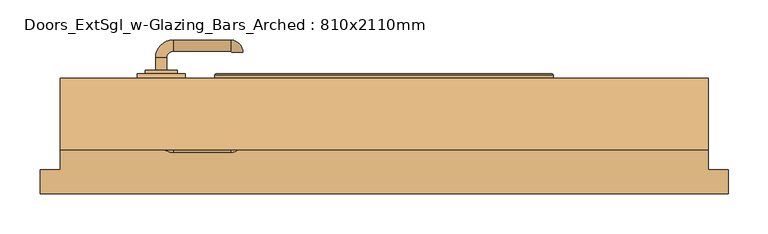
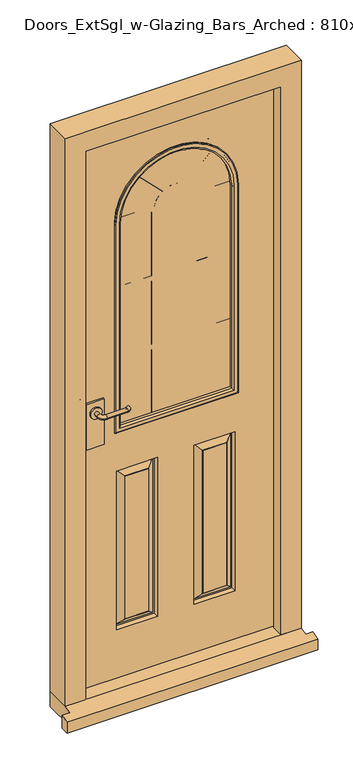
"""IFC4 building model written with IfcOpenShell, lengths in millimetres: door geometry, Doors_ExtSgl_w-Glazing_Bars_Arched : 810x2110mm."""

from ifc_helpers import new_model, si_unit, point, frame, frame_2d, origin, place, context, project, spatial, polyline, circle_curve, ellipse_curve, trimmed, segment, composite_curve, outline, extrude, faceted_brep, source, transform, mapped, element, save
from ifc_brep_helpers import plane_surface, cylinder_surface, revolved_surface, advanced_brep


def doors_extsgl_w_glazing_bars_arched_810x2110mm_84a0a083(model_context):
    return source(origin(), model_context, "Body", "SolidModel", [
        extrude(outline(composite_curve([segment(trimmed(circle_curve(frame_2d((1050.0, -278.5)), 20.0), [point((1050.0, -298.5))], [point((1050.0, -258.5))], False, "CARTESIAN"), True, "CONTINUOUS"), segment(trimmed(circle_curve(frame_2d((1050.0, -278.5)), 20.0), [point((1050.0, -258.5))], [point((1050.0, -298.5))], False, "CARTESIAN"), True, "CONTINUOUS")], self_intersect=False)), frame((0.0, 18.4, 0.0), z_axis=(0.0, 1.0, 0.0), x_axis=(0.0, 0.0, 1.0)), (0.0, 0.0, 1.0), 4.5929895),
        advanced_brep(
        [(-271.5, 22.9929895, 1050.0), (-285.5, 22.9929895, 1050.0), (-271.5, 38.4, 1050.0), (-285.5, 38.4, 1050.0), (-263.5, 60.4, 1050.0), (-263.5, 46.4, 1050.0), (-191.5, 46.4, 1050.0), (-191.5, 60.4, 1050.0), (-190.5, 45.4, 1050.0), (-176.5, 45.4, 1050.0)],
        [
            (0, 1, circle_curve(frame((-278.5, 22.9929895, 1050.0), z_axis=(0.0, -1.0, 0.0), x_axis=(-1.0, 0.0, 0.0)), 7.0)),
            (1, 0, circle_curve(frame((-278.5, 22.9929895, 1050.0), z_axis=(0.0, -1.0, 0.0), x_axis=(-1.0, 0.0, 0.0)), 7.0)),
            (0, 2),
            (2, 3, circle_curve(frame((-278.5, 38.4, 1050.0), z_axis=(0.0, -1.0, 0.0), x_axis=(-1.0, 0.0, 0.0)), 7.0)),
            (3, 1),
            (3, 2, circle_curve(frame((-278.5, 38.4, 1050.0), z_axis=(0.0, -1.0, 0.0), x_axis=(-1.0, 0.0, 0.0)), 7.0)),
            (4, 3, circle_curve(frame((-263.5, 38.4, 1050.0), z_axis=(0.0, 0.0, 1.0), x_axis=(-1.0, 0.0, 0.0)), 22.0)),
            (2, 5, circle_curve(frame((-263.5, 38.4, 1050.0), z_axis=(0.0, 0.0, -1.0), x_axis=(-1.0, 0.0, 0.0)), 8.0)),
            (5, 4, circle_curve(frame((-263.5, 53.4, 1050.0), z_axis=(-1.0, 0.0, 0.0), x_axis=(0.0, 1.0, 0.0)), 7.0)),
            (4, 5, circle_curve(frame((-263.5, 53.4, 1050.0), z_axis=(-1.0, 0.0, 0.0), x_axis=(0.0, 1.0, 0.0)), 7.0)),
            (5, 6),
            (6, 7, circle_curve(frame((-191.5, 53.4, 1050.0), z_axis=(-1.0, 0.0, 0.0), x_axis=(0.0, 1.0, 0.0)), 7.0)),
            (7, 4),
            (7, 6, circle_curve(frame((-191.5, 53.4, 1050.0), z_axis=(-1.0, 0.0, 0.0), x_axis=(0.0, 1.0, 0.0)), 7.0)),
            (8, 9, circle_curve(frame((-183.5, 45.4, 1050.0), z_axis=(0.0, -1.0, 0.0), x_axis=(1.0, 0.0, 0.0)), 7.0)),
            (9, 8, circle_curve(frame((-183.5, 45.4, 1050.0), z_axis=(0.0, -1.0, 0.0), x_axis=(1.0, 0.0, 0.0)), 7.0)),
            (9, 7, circle_curve(frame((-191.5, 45.4, 1050.0), z_axis=(0.0, 0.0, 1.0), x_axis=(0.0, 1.0, 0.0)), 15.0)),
            (6, 8, circle_curve(frame((-191.5, 45.4, 1050.0), z_axis=(0.0, 0.0, -1.0), x_axis=(0.0, 1.0, 0.0)), 1.0)),
        ],
        [
            plane_surface(frame((-278.5, 22.9929895, 1050.0), z_axis=(0.0, -1.0, 0.0), x_axis=(0.0, 0.0, 1.0))),
            cylinder_surface(frame((-278.5, 22.9929895, 1050.0), z_axis=(0.0, -1.0, 0.0), x_axis=(-1.0, 0.0, 0.0)), 7.0),
            revolved_surface(trimmed(ellipse_curve(frame((-278.5, 38.4, 1050.0), z_axis=(0.0, -1.0, 0.0), x_axis=(-1.0, 0.0, 0.0)), 7.0, 7.0), [point((-271.5, 38.4, 1050.0))], [point((-285.5, 38.4, 1050.0))], True, "CARTESIAN"), (-263.5, 38.4, 1050.0), (0.0, 0.0, -1.0)),
            revolved_surface(trimmed(ellipse_curve(frame((-278.5, 38.4, 1050.0), z_axis=(0.0, -1.0, 0.0), x_axis=(-1.0, 0.0, 0.0)), 7.0, 7.0), [point((-285.5, 38.4, 1050.0))], [point((-271.5, 38.4, 1050.0))], True, "CARTESIAN"), (-263.5, 38.4, 1050.0), (0.0, 0.0, -1.0)),
            cylinder_surface(frame((-263.5, 53.4, 1050.0), z_axis=(-1.0, 0.0, 0.0), x_axis=(0.0, 1.0, 0.0)), 7.0),
            plane_surface(frame((-183.5, 45.4, 1050.0), z_axis=(0.0, -1.0, 0.0), x_axis=(0.0, 0.0, 1.0))),
            revolved_surface(trimmed(ellipse_curve(frame((-191.5, 53.4, 1050.0), z_axis=(-1.0, 0.0, 0.0), x_axis=(0.0, 1.0, 0.0)), 7.0, 7.0), [point((-191.5, 46.4, 1050.0))], [point((-191.5, 60.4, 1050.0))], True, "CARTESIAN"), (-191.5, 45.4, 1050.0), (0.0, 0.0, -1.0)),
            revolved_surface(trimmed(ellipse_curve(frame((-191.5, 53.4, 1050.0), z_axis=(-1.0, 0.0, 0.0), x_axis=(0.0, 1.0, 0.0)), 7.0, 7.0), [point((-191.5, 60.4, 1050.0))], [point((-191.5, 46.4, 1050.0))], True, "CARTESIAN"), (-191.5, 45.4, 1050.0), (0.0, 0.0, -1.0)),
        ],
        [
            (0, [[1, 2]]),
            (1, [[-1, 3, 4, 5]]),
            (1, [[-2, -5, 6, -3]]),
            (2, [[7, -4, 8, 9]]),
            (3, [[-8, -6, -7, 10]]),
            (4, [[-9, 11, 12, 13]]),
            (4, [[-10, -13, 14, -11]]),
            (5, [[15, 16]]),
            (6, [[17, -12, 18, -16]]),
            (7, [[-18, -14, -17, -15]]),
        ],
    ),
        extrude(outline(polyline([(-248.5, 12.4), (-308.5, 12.4), (-308.5, 18.4), (-248.5, 18.4), (-248.5, 12.4)])), frame((0.0, 0.0, 925.0), z_axis=(0.0, 0.0, 1.0), x_axis=(1.0, 0.0, 0.0)), (0.0, 0.0, 1.0), 165.0),
        extrude(outline(composite_curve([segment(trimmed(circle_curve(frame_2d((1050.0, -278.5)), 20.0), [point((1050.0, -298.5))], [point((1050.0, -258.5))], False, "CARTESIAN"), True, "CONTINUOUS"), segment(trimmed(circle_curve(frame_2d((1050.0, -278.5)), 20.0), [point((1050.0, -258.5))], [point((1050.0, -298.5))], False, "CARTESIAN"), True, "CONTINUOUS")], self_intersect=False)), frame((0.0, -42.1929895, 0.0), z_axis=(0.0, 1.0, 0.0), x_axis=(0.0, 0.0, 1.0)), (0.0, 0.0, 1.0), 4.5929895),
        advanced_brep(
        [(-271.5, -42.1929895, 1050.0), (-285.5, -42.1929895, 1050.0), (-285.5, -57.6, 1050.0), (-271.5, -57.6, 1050.0), (-263.5, -79.6, 1050.0), (-263.5, -65.6, 1050.0), (-191.5, -79.6, 1050.0), (-191.5, -65.6, 1050.0), (-190.5, -64.6, 1050.0), (-176.5, -64.6, 1050.0)],
        [
            (0, 1, circle_curve(frame((-278.5, -42.1929895, 1050.0), z_axis=(0.0, 1.0, 0.0), x_axis=(-1.0, 0.0, 0.0)), 7.0)),
            (1, 0, circle_curve(frame((-278.5, -42.1929895, 1050.0), z_axis=(0.0, 1.0, 0.0), x_axis=(-1.0, 0.0, 0.0)), 7.0)),
            (1, 2),
            (2, 3, circle_curve(frame((-278.5, -57.6, 1050.0), z_axis=(0.0, 1.0, 0.0), x_axis=(-1.0, 0.0, 0.0)), 7.0)),
            (3, 0),
            (3, 2, circle_curve(frame((-278.5, -57.6, 1050.0), z_axis=(0.0, 1.0, 0.0), x_axis=(-1.0, 0.0, 0.0)), 7.0)),
            (4, 5, circle_curve(frame((-263.5, -72.6, 1050.0), z_axis=(-1.0, 0.0, 0.0), x_axis=(0.0, -1.0, 0.0)), 7.0)),
            (5, 3, circle_curve(frame((-263.5, -57.6, 1050.0), z_axis=(0.0, 0.0, -1.0), x_axis=(-1.0, 0.0, 0.0)), 8.0)),
            (2, 4, circle_curve(frame((-263.5, -57.6, 1050.0), z_axis=(0.0, 0.0, 1.0), x_axis=(-1.0, 0.0, 0.0)), 22.0)),
            (5, 4, circle_curve(frame((-263.5, -72.6, 1050.0), z_axis=(-1.0, 0.0, 0.0), x_axis=(0.0, -1.0, 0.0)), 7.0)),
            (4, 6),
            (6, 7, circle_curve(frame((-191.5, -72.6, 1050.0), z_axis=(-1.0, 0.0, 0.0), x_axis=(0.0, -1.0, 0.0)), 7.0)),
            (7, 5),
            (7, 6, circle_curve(frame((-191.5, -72.6, 1050.0), z_axis=(-1.0, 0.0, 0.0), x_axis=(0.0, -1.0, 0.0)), 7.0)),
            (8, 9, circle_curve(frame((-183.5, -64.6, 1050.0), z_axis=(0.0, 1.0, 0.0), x_axis=(1.0, 0.0, 0.0)), 7.0)),
            (9, 8, circle_curve(frame((-183.5, -64.6, 1050.0), z_axis=(0.0, 1.0, 0.0), x_axis=(1.0, 0.0, 0.0)), 7.0)),
            (8, 7, circle_curve(frame((-191.5, -64.6, 1050.0), z_axis=(0.0, 0.0, -1.0), x_axis=(0.0, -1.0, 0.0)), 1.0)),
            (6, 9, circle_curve(frame((-191.5, -64.6, 1050.0), z_axis=(0.0, 0.0, 1.0), x_axis=(0.0, -1.0, 0.0)), 15.0)),
        ],
        [
            plane_surface(frame((-278.5, -42.1929895, 1050.0), z_axis=(0.0, 1.0, 0.0), x_axis=(0.0, 0.0, 1.0))),
            cylinder_surface(frame((-278.5, -42.1929895, 1050.0), z_axis=(0.0, 1.0, 0.0), x_axis=(-1.0, 0.0, 0.0)), 7.0),
            revolved_surface(trimmed(ellipse_curve(frame((-278.5, -57.6, 1050.0), z_axis=(0.0, -1.0, 0.0), x_axis=(-1.0, 0.0, 0.0)), 7.0, 7.0), [point((-271.5, -57.6, 1050.0))], [point((-285.5, -57.6, 1050.0))], True, "CARTESIAN"), (-263.5, -57.6, 1050.0), (0.0, 0.0, -1.0)),
            revolved_surface(trimmed(ellipse_curve(frame((-278.5, -57.6, 1050.0), z_axis=(0.0, -1.0, 0.0), x_axis=(-1.0, 0.0, 0.0)), 7.0, 7.0), [point((-285.5, -57.6, 1050.0))], [point((-271.5, -57.6, 1050.0))], True, "CARTESIAN"), (-263.5, -57.6, 1050.0), (0.0, 0.0, -1.0)),
            cylinder_surface(frame((-263.5, -72.6, 1050.0), z_axis=(-1.0, 0.0, 0.0), x_axis=(0.0, -1.0, 0.0)), 7.0),
            plane_surface(frame((-183.5, -64.6, 1050.0), z_axis=(0.0, 1.0, 0.0), x_axis=(0.0, 0.0, 1.0))),
            revolved_surface(trimmed(ellipse_curve(frame((-191.5, -72.6, 1050.0), z_axis=(1.0, 0.0, 0.0), x_axis=(0.0, -1.0, 0.0)), 7.0, 7.0), [point((-191.5, -65.6, 1050.0))], [point((-191.5, -79.6, 1050.0))], True, "CARTESIAN"), (-191.5, -64.6, 1050.0), (0.0, 0.0, -1.0)),
            revolved_surface(trimmed(ellipse_curve(frame((-191.5, -72.6, 1050.0), z_axis=(1.0, 0.0, 0.0), x_axis=(0.0, -1.0, 0.0)), 7.0, 7.0), [point((-191.5, -79.6, 1050.0))], [point((-191.5, -65.6, 1050.0))], True, "CARTESIAN"), (-191.5, -64.6, 1050.0), (0.0, 0.0, -1.0)),
        ],
        [
            (0, [[1, 2]]),
            (1, [[3, 4, 5, -2]]),
            (1, [[-5, 6, -3, -1]]),
            (2, [[7, 8, -4, 9]]),
            (3, [[10, -9, -6, -8]]),
            (4, [[11, 12, 13, -7]]),
            (4, [[-13, 14, -11, -10]]),
            (5, [[15, 16]]),
            (6, [[-15, 17, -12, 18]]),
            (7, [[-16, -18, -14, -17]]),
        ],
    ),
        extrude(outline(polyline([(-248.5, -31.6), (-248.5, -37.6), (-308.5, -37.6), (-308.5, -31.6), (-248.5, -31.6)])), frame((0.0, 0.0, 925.0), z_axis=(0.0, 0.0, 1.0), x_axis=(1.0, 0.0, 0.0)), (0.0, 0.0, 1.0), 165.0),
        faceted_brep([(334.5, -76.6, 54.5), (334.5, -34.6, 54.5), (356.5, -34.6, 54.5), (356.5, 12.4, 54.5), (405.0, 12.4, 54.5), (405.0, -76.6, 54.5), (405.0, -76.6, 2110.0), (-405.0, -76.6, 2110.0), (-405.0, -76.6, 54.5), (-334.5, -76.6, 54.5), (-334.5, -76.6, 2039.5), (334.5, -76.6, 2039.5), (405.0, 12.4, 2110.0), (356.5, 12.4, 2061.5), (-356.5, 12.4, 2061.5), (-356.5, 12.4, 54.5), (-405.0, 12.4, 54.5), (-405.0, 12.4, 2110.0), (356.5, -34.6, 2061.5), (334.5, -34.6, 2039.5), (-334.5, -34.6, 2039.5), (-334.5, -34.6, 54.5), (-356.5, -34.6, 54.5), (-356.5, -34.6, 2061.5)], [[[0, 1, 2, 3, 4, 5]], [[5, 6, 7, 8, 9, 10, 11, 0]], [[4, 12, 6, 5]], [[3, 13, 14, 15, 16, 17, 12, 4]], [[2, 18, 13, 3]], [[1, 19, 20, 21, 22, 23, 18, 2]], [[0, 11, 19, 1]], [[9, 21, 20, 10]], [[8, 16, 15, 22, 21, 9]], [[7, 17, 16, 8]], [[14, 23, 22, 15]], [[6, 12, 17, 7]], [[13, 18, 23, 14]], [[10, 20, 19, 11]]]),
        advanced_brep(
        [(353.5, 12.4, 58.5), (-354.4250294, 12.4, 58.5), (-354.4250294, 12.4, 2058.5), (353.5, 12.4, 2058.5), (-203.5, 12.4, 958.5), (203.5, 12.4, 958.5), (203.5, 12.4, 1705.0), (-203.5, 12.4, 1705.0), (-62.5, 12.4, 808.5), (-203.5, 12.4, 808.5), (-203.5, 12.4, 233.5), (-62.5, 12.4, 233.5), (203.5, 12.4, 808.5), (62.5, 12.4, 808.5), (62.5, 12.4, 233.5), (203.5, 12.4, 233.5), (-92.5, 12.4, 263.5), (-173.5, 12.4, 263.5), (-173.5, 12.4, 778.5), (-92.5, 12.4, 778.5), (173.5, 12.4, 263.5), (92.5, 12.4, 263.5), (92.5, 12.4, 778.5), (173.5, 12.4, 778.5), (353.5, -31.6, 58.5), (353.5, -31.6, 2058.5), (-354.4250294, -31.6, 2058.5), (-354.4250294, -31.6, 58.5), (-203.5, -31.6, 958.5), (-203.5, -31.6, 1705.0), (203.5, -31.6, 1705.0), (203.5, -31.6, 958.5), (62.5, -31.6, 808.5), (203.5, -31.6, 808.5), (203.5, -31.6, 233.5), (62.5, -31.6, 233.5), (-203.5, -31.6, 808.5), (-62.5, -31.6, 808.5), (-62.5, -31.6, 233.5), (-203.5, -31.6, 233.5), (92.5, -31.6, 263.5), (173.5, -31.6, 263.5), (173.5, -31.6, 778.5), (92.5, -31.6, 778.5), (-173.5, -31.6, 263.5), (-92.5, -31.6, 263.5), (-92.5, -31.6, 778.5), (-173.5, -31.6, 778.5), (65.5, -16.6, 805.5), (65.5, -16.6, 236.5), (90.5, -30.6, 780.5), (70.5, -16.6, 800.5), (70.5, -16.6, 241.5), (90.5, -30.6, 261.5), (92.5, -30.6, 778.5), (92.5, -30.6, 263.5), (200.5, -16.6, 236.5), (195.5, -16.6, 241.5), (175.5, -30.6, 261.5), (173.5, -30.6, 263.5), (200.5, -16.6, 805.5), (195.5, -16.6, 800.5), (175.5, -30.6, 780.5), (173.5, -30.6, 778.5), (-200.5, -16.6, 805.5), (-200.5, -16.6, 236.5), (-175.5, -30.6, 780.5), (-195.5, -16.6, 800.5), (-195.5, -16.6, 241.5), (-175.5, -30.6, 261.5), (-173.5, -30.6, 778.5), (-173.5, -30.6, 263.5), (-65.5, -16.6, 236.5), (-70.5, -16.6, 241.5), (-90.5, -30.6, 261.5), (-92.5, -30.6, 263.5), (-65.5, -16.6, 805.5), (-70.5, -16.6, 800.5), (-90.5, -30.6, 780.5), (-92.5, -30.6, 778.5), (-92.5, 11.4, 263.5), (-92.5, 11.4, 778.5), (-70.5, -2.6, 241.5), (-90.5, 11.4, 261.5), (-90.5, 11.4, 780.5), (-70.5, -2.6, 800.5), (-65.5, -2.6, 236.5), (-65.5, -2.6, 805.5), (-173.5, 11.4, 778.5), (-175.5, 11.4, 780.5), (-195.5, -2.6, 800.5), (-200.5, -2.6, 805.5), (-173.5, 11.4, 263.5), (-175.5, 11.4, 261.5), (-195.5, -2.6, 241.5), (-200.5, -2.6, 236.5), (200.5, -2.6, 805.5), (200.5, -2.6, 236.5), (175.5, 11.4, 780.5), (195.5, -2.6, 800.5), (195.5, -2.6, 241.5), (175.5, 11.4, 261.5), (173.5, 11.4, 778.5), (173.5, 11.4, 263.5), (65.5, -2.6, 236.5), (70.5, -2.6, 241.5), (90.5, 11.4, 261.5), (92.5, 11.4, 263.5), (65.5, -2.6, 805.5), (70.5, -2.6, 800.5), (90.5, 11.4, 780.5), (92.5, 11.4, 778.5)],
        [
            (0, 1),
            (1, 2),
            (2, 3),
            (3, 0),
            (4, 5),
            (5, 6),
            (6, 7, circle_curve(frame((0.0, 12.4, 1705.0), z_axis=(0.0, -1.0, 0.0), x_axis=(1.0, 0.0, 0.0)), 203.5)),
            (7, 4),
            (8, 9),
            (9, 10),
            (10, 11),
            (11, 8),
            (12, 13),
            (13, 14),
            (14, 15),
            (15, 12),
            (16, 17),
            (17, 18),
            (18, 19),
            (19, 16),
            (20, 21),
            (21, 22),
            (22, 23),
            (23, 20),
            (24, 25),
            (25, 26),
            (26, 27),
            (27, 24),
            (28, 29),
            (29, 30, circle_curve(frame((0.0, -31.6, 1705.0), z_axis=(0.0, 1.0, 0.0), x_axis=(1.0, 0.0, 0.0)), 203.5)),
            (30, 31),
            (31, 28),
            (32, 33),
            (33, 34),
            (34, 35),
            (35, 32),
            (36, 37),
            (37, 38),
            (38, 39),
            (39, 36),
            (40, 41),
            (41, 42),
            (42, 43),
            (43, 40),
            (44, 45),
            (45, 46),
            (46, 47),
            (47, 44),
            (3, 25),
            (24, 0),
            (2, 26),
            (1, 27),
            (7, 29),
            (28, 4),
            (6, 30),
            (5, 31),
            (48, 32),
            (35, 49),
            (49, 48),
            (50, 51),
            (51, 52),
            (52, 53),
            (53, 50),
            (43, 54),
            (54, 55),
            (55, 40),
            (34, 56),
            (56, 49),
            (52, 57),
            (57, 58),
            (58, 53),
            (55, 59),
            (59, 41),
            (33, 60),
            (60, 56),
            (57, 61),
            (61, 62),
            (62, 58),
            (59, 63),
            (63, 42),
            (48, 60),
            (51, 61),
            (50, 62),
            (54, 63),
            (64, 36),
            (39, 65),
            (65, 64),
            (66, 67),
            (67, 68),
            (68, 69),
            (69, 66),
            (47, 70),
            (70, 71),
            (71, 44),
            (38, 72),
            (72, 65),
            (68, 73),
            (73, 74),
            (74, 69),
            (71, 75),
            (75, 45),
            (37, 76),
            (76, 72),
            (73, 77),
            (77, 78),
            (78, 74),
            (75, 79),
            (79, 46),
            (64, 76),
            (67, 77),
            (66, 78),
            (70, 79),
            (80, 16),
            (19, 81),
            (81, 80),
            (82, 83),
            (83, 84),
            (84, 85),
            (85, 82),
            (11, 86),
            (86, 87),
            (87, 8),
            (18, 88),
            (88, 81),
            (84, 89),
            (89, 90),
            (90, 85),
            (87, 91),
            (91, 9),
            (17, 92),
            (92, 88),
            (89, 93),
            (93, 94),
            (94, 90),
            (91, 95),
            (95, 10),
            (80, 92),
            (83, 93),
            (82, 94),
            (86, 95),
            (96, 12),
            (15, 97),
            (97, 96),
            (98, 99),
            (99, 100),
            (100, 101),
            (101, 98),
            (23, 102),
            (102, 103),
            (103, 20),
            (14, 104),
            (104, 97),
            (100, 105),
            (105, 106),
            (106, 101),
            (103, 107),
            (107, 21),
            (13, 108),
            (108, 104),
            (105, 109),
            (109, 110),
            (110, 106),
            (107, 111),
            (111, 22),
            (96, 108),
            (99, 109),
            (98, 110),
            (102, 111),
        ],
        [
            plane_surface(frame((353.5, 12.4, 58.5), z_axis=(0.0, 1.0, 0.0), x_axis=(0.0, 0.0, 1.0))),
            plane_surface(frame((353.5, -31.6, 58.5), z_axis=(0.0, -1.0, 0.0), x_axis=(0.0, 0.0, -1.0))),
            plane_surface(frame((353.5, 12.4, 58.5), z_axis=(1.0, 0.0, 0.0), x_axis=(0.0, -1.0, 0.0))),
            plane_surface(frame((353.5, 12.4, 2058.5), z_axis=(0.0, 0.0, 1.0), x_axis=(0.0, -1.0, 0.0))),
            plane_surface(frame((-354.4250294, 12.4, 2058.5), z_axis=(-1.0, 0.0, 0.0), x_axis=(0.0, -1.0, 0.0))),
            plane_surface(frame((-354.4250294, 12.4, 58.5), z_axis=(0.0, 0.0, -1.0), x_axis=(0.0, -1.0, 0.0))),
            plane_surface(frame((-203.5, 12.4, 958.5), z_axis=(1.0, 0.0, 0.0), x_axis=(0.0, -1.0, 0.0))),
            revolved_surface(polyline([(203.5, -31.6, 1705.0), (203.5, 12.4, 1705.0)]), (0.0, 12.4, 1705.0), (0.0, -1.0, 0.0)),
            plane_surface(frame((203.5, 12.4, 1705.0), z_axis=(-1.0, 0.0, 0.0), x_axis=(0.0, -1.0, 0.0))),
            plane_surface(frame((203.5, 12.4, 958.5), z_axis=(0.0, 0.0, 1.0), x_axis=(0.0, -1.0, 0.0))),
            plane_surface(frame((62.5, -31.6, 808.5), z_axis=(0.9805806756909202, -0.19611613513818407, 0.0), x_axis=(0.0, 0.0, -1.0))),
            plane_surface(frame((70.5, -16.6, 800.5), z_axis=(-0.5734623443633278, -0.8192319205190408, 0.0), x_axis=(0.0, 0.0, -1.0))),
            plane_surface(frame((92.5, -30.6, 778.5), z_axis=(-1.0, 0.0, 0.0), x_axis=(0.0, 0.0, -1.0))),
            plane_surface(frame((62.5, -31.6, 233.5), z_axis=(0.0, -0.19611613513818718, 0.9805806756909196), x_axis=(1.0, 0.0, 0.0))),
            plane_surface(frame((70.5, -16.6, 241.5), z_axis=(0.0, -0.8192319205190389, -0.5734623443633305), x_axis=(1.0, 0.0, 0.0))),
            plane_surface(frame((92.5, -30.6, 263.5), z_axis=(0.0, 0.0, -1.0), x_axis=(1.0, 0.0, 0.0))),
            plane_surface(frame((203.5, -31.6, 233.5), z_axis=(-0.9805806756909189, -0.19611613513819035, 0.0), x_axis=(0.0, 0.0, 1.0))),
            plane_surface(frame((195.5, -16.6, 241.5), z_axis=(0.5734623443633332, -0.819231920519037, 0.0), x_axis=(0.0, 0.0, 1.0))),
            plane_surface(frame((173.5, -30.6, 263.5), z_axis=(1.0, 0.0, 0.0), x_axis=(0.0, 0.0, 1.0))),
            plane_surface(frame((203.5, -31.6, 808.5), z_axis=(0.0, -0.19611613513818718, -0.9805806756909196), x_axis=(-1.0, 0.0, 0.0))),
            plane_surface(frame((200.5, -16.6, 805.5), z_axis=(0.0, -1.0, 0.0), x_axis=(-1.0, 0.0, 0.0))),
            plane_surface(frame((195.5, -16.6, 800.5), z_axis=(0.0, -0.8192319205190389, 0.5734623443633305), x_axis=(-1.0, 0.0, 0.0))),
            plane_surface(frame((175.5, -30.6, 780.5), z_axis=(0.0, -1.0, 0.0), x_axis=(-1.0, 0.0, 0.0))),
            plane_surface(frame((173.5, -30.6, 778.5), z_axis=(0.0, 0.0, 1.0), x_axis=(-1.0, 0.0, 0.0))),
            plane_surface(frame((-203.5, -31.6, 808.5), z_axis=(0.9805806756909202, -0.19611613513818407, 0.0), x_axis=(0.0, 0.0, -1.0))),
            plane_surface(frame((-195.5, -16.6, 800.5), z_axis=(-0.5734623443633278, -0.8192319205190408, 0.0), x_axis=(0.0, 0.0, -1.0))),
            plane_surface(frame((-173.5, -30.6, 778.5), z_axis=(-1.0, 0.0, 0.0), x_axis=(0.0, 0.0, -1.0))),
            plane_surface(frame((-203.5, -31.6, 233.5), z_axis=(0.0, -0.19611613513818724, 0.9805806756909196), x_axis=(1.0, 0.0, 0.0))),
            plane_surface(frame((-195.5, -16.6, 241.5), z_axis=(0.0, -0.819231920519039, -0.5734623443633305), x_axis=(1.0, 0.0, 0.0))),
            plane_surface(frame((-173.5, -30.6, 263.5), z_axis=(0.0, 0.0, -1.0), x_axis=(1.0, 0.0, 0.0))),
            plane_surface(frame((-62.5, -31.6, 233.5), z_axis=(-0.9805806756909189, -0.1961161351381904, 0.0), x_axis=(0.0, 0.0, 1.0))),
            plane_surface(frame((-70.5, -16.6, 241.5), z_axis=(0.5734623443633332, -0.8192319205190371, 0.0), x_axis=(0.0, 0.0, 1.0))),
            plane_surface(frame((-92.5, -30.6, 263.5), z_axis=(1.0, 0.0, 0.0), x_axis=(0.0, 0.0, 1.0))),
            plane_surface(frame((-62.5, -31.6, 808.5), z_axis=(0.0, -0.19611613513818724, -0.9805806756909196), x_axis=(-1.0, 0.0, 0.0))),
            plane_surface(frame((-65.5, -16.6, 805.5), z_axis=(0.0, -1.0, 0.0), x_axis=(-1.0, 0.0, 0.0))),
            plane_surface(frame((-70.5, -16.6, 800.5), z_axis=(0.0, -0.819231920519039, 0.5734623443633305), x_axis=(-1.0, 0.0, 0.0))),
            plane_surface(frame((-90.5, -30.6, 780.5), z_axis=(0.0, -1.0, 0.0), x_axis=(-1.0, 0.0, 0.0))),
            plane_surface(frame((-92.5, -30.6, 778.5), z_axis=(0.0, 0.0, 1.0), x_axis=(-1.0, 0.0, 0.0))),
            plane_surface(frame((-92.5, 12.4, 263.5), z_axis=(1.0, 0.0, 0.0), x_axis=(0.0, 0.0, 1.0))),
            plane_surface(frame((-90.5, 11.4, 261.5), z_axis=(0.5734623443633226, 0.8192319205190445, 0.0), x_axis=(0.0, 0.0, 1.0))),
            plane_surface(frame((-65.5, -2.6, 236.5), z_axis=(-0.9805806756909214, 0.1961161351381777, 0.0), x_axis=(0.0, 0.0, 1.0))),
            plane_surface(frame((-92.5, 12.4, 778.5), z_axis=(0.0, 0.0, 1.0), x_axis=(-1.0, 0.0, 0.0))),
            plane_surface(frame((-90.5, 11.4, 780.5), z_axis=(0.0, 0.8192319205190427, 0.5734623443633253), x_axis=(-1.0, 0.0, 0.0))),
            plane_surface(frame((-65.5, -2.6, 805.5), z_axis=(0.0, 0.19611613513818085, -0.9805806756909208), x_axis=(-1.0, 0.0, 0.0))),
            plane_surface(frame((-173.5, 12.4, 778.5), z_axis=(-1.0, 0.0, 0.0), x_axis=(0.0, 0.0, -1.0))),
            plane_surface(frame((-175.5, 11.4, 780.5), z_axis=(-0.5734623443633281, 0.8192319205190407, 0.0), x_axis=(0.0, 0.0, -1.0))),
            plane_surface(frame((-200.5, -2.6, 805.5), z_axis=(0.9805806756909202, 0.196116135138184, 0.0), x_axis=(0.0, 0.0, -1.0))),
            plane_surface(frame((-173.5, 12.4, 263.5), z_axis=(0.0, 0.0, -1.0), x_axis=(1.0, 0.0, 0.0))),
            plane_surface(frame((-173.5, 11.4, 263.5), z_axis=(0.0, 1.0, 0.0), x_axis=(1.0, 0.0, 0.0))),
            plane_surface(frame((-175.5, 11.4, 261.5), z_axis=(0.0, 0.8192319205190426, -0.5734623443633253), x_axis=(1.0, 0.0, 0.0))),
            plane_surface(frame((-195.5, -2.6, 241.5), z_axis=(0.0, 1.0, 0.0), x_axis=(1.0, 0.0, 0.0))),
            plane_surface(frame((-200.5, -2.6, 236.5), z_axis=(0.0, 0.19611613513818088, 0.9805806756909209), x_axis=(1.0, 0.0, 0.0))),
            plane_surface(frame((203.5, 12.4, 808.5), z_axis=(-0.9805806756909202, 0.19611613513818407, 0.0), x_axis=(0.0, 0.0, -1.0))),
            plane_surface(frame((195.5, -2.6, 800.5), z_axis=(0.5734623443633278, 0.8192319205190408, 0.0), x_axis=(0.0, 0.0, -1.0))),
            plane_surface(frame((173.5, 11.4, 778.5), z_axis=(1.0, 0.0, 0.0), x_axis=(0.0, 0.0, -1.0))),
            plane_surface(frame((203.5, 12.4, 233.5), z_axis=(0.0, 0.19611613513818724, 0.9805806756909196), x_axis=(-1.0, 0.0, 0.0))),
            plane_surface(frame((195.5, -2.6, 241.5), z_axis=(0.0, 0.819231920519039, -0.5734623443633305), x_axis=(-1.0, 0.0, 0.0))),
            plane_surface(frame((173.5, 11.4, 263.5), z_axis=(0.0, 0.0, -1.0), x_axis=(-1.0, 0.0, 0.0))),
            plane_surface(frame((62.5, 12.4, 233.5), z_axis=(0.9805806756909189, 0.19611613513819046, 0.0), x_axis=(0.0, 0.0, 1.0))),
            plane_surface(frame((70.5, -2.6, 241.5), z_axis=(-0.5734623443633331, 0.8192319205190371, 0.0), x_axis=(0.0, 0.0, 1.0))),
            plane_surface(frame((92.5, 11.4, 263.5), z_axis=(-1.0, 0.0, 0.0), x_axis=(0.0, 0.0, 1.0))),
            plane_surface(frame((62.5, 12.4, 808.5), z_axis=(0.0, 0.19611613513818724, -0.9805806756909196), x_axis=(1.0, 0.0, 0.0))),
            plane_surface(frame((65.5, -2.6, 805.5), z_axis=(0.0, 1.0, 0.0), x_axis=(1.0, 0.0, 0.0))),
            plane_surface(frame((70.5, -2.6, 800.5), z_axis=(0.0, 0.819231920519039, 0.5734623443633305), x_axis=(1.0, 0.0, 0.0))),
            plane_surface(frame((90.5, 11.4, 780.5), z_axis=(0.0, 1.0, 0.0), x_axis=(1.0, 0.0, 0.0))),
            plane_surface(frame((92.5, 11.4, 778.5), z_axis=(0.0, 0.0, 1.0), x_axis=(1.0, 0.0, 0.0))),
        ],
        [
            (0, [[1, 2, 3, 4], [5, 6, 7, 8], [9, 10, 11, 12], [13, 14, 15, 16]]),
            (0, [[17, 18, 19, 20]]),
            (0, [[21, 22, 23, 24]]),
            (1, [[25, 26, 27, 28], [29, 30, 31, 32], [33, 34, 35, 36], [37, 38, 39, 40]]),
            (1, [[41, 42, 43, 44]]),
            (1, [[45, 46, 47, 48]]),
            (2, [[49, -25, 50, -4]]),
            (3, [[51, -26, -49, -3]]),
            (4, [[52, -27, -51, -2]]),
            (5, [[-50, -28, -52, -1]]),
            (6, [[53, -29, 54, -8]]),
            (7, [[55, -30, -53, -7]]),
            (8, [[56, -31, -55, -6]]),
            (9, [[-54, -32, -56, -5]]),
            (10, [[57, -36, 58, 59]]),
            (11, [[60, 61, 62, 63]]),
            (12, [[-44, 64, 65, 66]]),
            (13, [[-35, 67, 68, -58]]),
            (14, [[69, 70, 71, -62]]),
            (15, [[72, 73, -41, -66]]),
            (16, [[-34, 74, 75, -67]]),
            (17, [[76, 77, 78, -70]]),
            (18, [[79, 80, -42, -73]]),
            (19, [[81, -74, -33, -57]]),
            (20, [[-68, -75, -81, -59], [82, -76, -69, -61]]),
            (21, [[83, -77, -82, -60]]),
            (22, [[-71, -78, -83, -63], [84, -79, -72, -65]]),
            (23, [[-43, -80, -84, -64]]),
            (24, [[85, -40, 86, 87]]),
            (25, [[88, 89, 90, 91]]),
            (26, [[-48, 92, 93, 94]]),
            (27, [[-39, 95, 96, -86]]),
            (28, [[97, 98, 99, -90]]),
            (29, [[100, 101, -45, -94]]),
            (30, [[-38, 102, 103, -95]]),
            (31, [[104, 105, 106, -98]]),
            (32, [[107, 108, -46, -101]]),
            (33, [[109, -102, -37, -85]]),
            (34, [[-96, -103, -109, -87], [110, -104, -97, -89]]),
            (35, [[111, -105, -110, -88]]),
            (36, [[-99, -106, -111, -91], [112, -107, -100, -93]]),
            (37, [[-47, -108, -112, -92]]),
            (38, [[113, -20, 114, 115]]),
            (39, [[116, 117, 118, 119]]),
            (40, [[-12, 120, 121, 122]]),
            (41, [[-19, 123, 124, -114]]),
            (42, [[125, 126, 127, -118]]),
            (43, [[128, 129, -9, -122]]),
            (44, [[-18, 130, 131, -123]]),
            (45, [[132, 133, 134, -126]]),
            (46, [[135, 136, -10, -129]]),
            (47, [[137, -130, -17, -113]]),
            (48, [[138, -132, -125, -117], [-124, -131, -137, -115]]),
            (49, [[139, -133, -138, -116]]),
            (50, [[140, -135, -128, -121], [-127, -134, -139, -119]]),
            (51, [[-11, -136, -140, -120]]),
            (52, [[141, -16, 142, 143]]),
            (53, [[144, 145, 146, 147]]),
            (54, [[-24, 148, 149, 150]]),
            (55, [[-15, 151, 152, -142]]),
            (56, [[153, 154, 155, -146]]),
            (57, [[156, 157, -21, -150]]),
            (58, [[-14, 158, 159, -151]]),
            (59, [[160, 161, 162, -154]]),
            (60, [[163, 164, -22, -157]]),
            (61, [[165, -158, -13, -141]]),
            (62, [[-152, -159, -165, -143], [166, -160, -153, -145]]),
            (63, [[167, -161, -166, -144]]),
            (64, [[-155, -162, -167, -147], [168, -163, -156, -149]]),
            (65, [[-23, -164, -168, -148]]),
        ],
    ),
        faceted_brep([(430.0, -131.6, 0.0), (430.0, -101.6, 0.0), (430.0, -101.6, 47.2703282), (430.0, -131.6, 38.5947221), (-430.0, -131.6, 38.5947221), (-430.0, -101.6, 47.2703282), (-430.0, -101.6, 0.0), (-430.0, -131.6, 0.0), (-405.0, -101.6, 0.0), (-405.0, 12.4, 0.0), (405.0, 12.4, 0.0), (405.0, -101.6, 0.0), (405.0, -101.6, 47.2703282), (405.0, -76.6, 54.5), (-405.0, -76.6, 54.5), (-405.0, -101.6, 47.2703282), (405.0, 12.4, 54.5), (-405.0, 12.4, 54.5)], [[[0, 1, 2, 3]], [[4, 5, 6, 7]], [[7, 6, 8, 9, 10, 11, 1, 0]], [[3, 4, 7, 0]], [[3, 2, 12, 13, 14, 15, 5, 4]], [[14, 13, 16, 17]], [[17, 16, 10, 9]], [[15, 14, 17, 9, 8]], [[8, 6, 5, 15]], [[11, 10, 16, 13, 12]], [[12, 2, 1, 11]]]),
        extrude(outline(composite_curve([segment(polyline([(958.5, -203.5), (958.5, 203.5), (1705.0, 203.5)]), True, "CONTINUOUS"), segment(trimmed(circle_curve(frame_2d((1705.0, 0.0)), 203.5), [point((1705.0, 203.5))], [point((1705.0, -203.5))], False, "CARTESIAN"), True, "CONTINUOUS"), segment(polyline([(1705.0, -203.5), (958.5, -203.5)]), True, "CONTINUOUS")], self_intersect=False)), frame((0.0, -21.6, 0.0), z_axis=(0.0, 1.0, 0.0), x_axis=(0.0, 0.0, 1.0)), (0.0, 0.0, 1.0), 24.0),
        advanced_brep(
        [(-211.5, -35.6, 950.5), (-211.5, -35.6, 1705.0), (-211.5, -31.6, 1705.0), (-211.5, -31.6, 950.5), (-209.5, -37.6, 952.5), (-209.5, -37.6, 1705.0), (-191.5, -32.6, 970.5), (-191.5, -32.6, 1705.0), (-196.5, -37.6, 1705.0), (-196.5, -37.6, 965.5), (-191.5, -21.6, 970.5), (-191.5, -21.6, 1705.0), (-203.5, -31.6, 958.5), (-203.5, -31.6, 1705.0), (-203.5, -21.6, 1705.0), (-203.5, -21.6, 958.5), (211.5, -35.6, 1705.0), (211.5, -31.6, 1705.0), (209.5, -37.6, 1705.0), (209.5, -37.6, 952.5), (196.5, -37.6, 1705.0), (196.5, -37.6, 965.5), (191.5, -32.6, 1705.0), (191.5, -21.6, 1705.0), (203.5, -21.6, 1705.0), (203.5, -21.6, 958.5), (191.5, -21.6, 970.5), (203.5, -31.6, 1705.0), (211.5, -31.6, 950.5), (203.5, -31.6, 958.5), (211.5, -35.6, 950.5), (191.5, -32.6, 970.5)],
        [
            (0, 1),
            (1, 2),
            (2, 3),
            (3, 0),
            (4, 5),
            (5, 1, circle_curve(frame((-209.5, -35.6, 1705.0), z_axis=(0.0, 0.0, -1.0), x_axis=(-1.0, 0.0, 0.0)), 2.0)),
            (0, 4, ellipse_curve(frame((-209.5, -35.6, 952.5), z_axis=(-0.7071067811865475, 0.0, 0.7071067811865475), x_axis=(-0.7071067811865472, 0.0, -0.7071067811865477)), 2.8284271, 2.0)),
            (6, 7),
            (7, 8, circle_curve(frame((-196.5, -32.6, 1705.0), z_axis=(0.0, 0.0, -1.0), x_axis=(-1.0, 0.0, 0.0)), 5.0)),
            (8, 9),
            (9, 6, ellipse_curve(frame((-196.5, -32.6, 965.5), z_axis=(-0.7071067811865475, 0.0, 0.7071067811865475), x_axis=(-0.7071067811865472, 0.0, -0.7071067811865477)), 7.0710678, 5.0)),
            (10, 11),
            (11, 7),
            (6, 10),
            (12, 13),
            (13, 14),
            (14, 15),
            (15, 12),
            (16, 17),
            (17, 2, circle_curve(frame((0.0, -31.6, 1705.0), z_axis=(0.0, -1.0, 0.0), x_axis=(-1.0, 0.0, 0.0)), 211.5)),
            (1, 16, circle_curve(frame((0.0, -35.6, 1705.0), z_axis=(0.0, 1.0, 0.0), x_axis=(-1.0, 0.0, 0.0)), 211.5)),
            (18, 16, circle_curve(frame((209.5, -35.6, 1705.0), z_axis=(0.0, 0.0, 1.0), x_axis=(1.0, 0.0, 0.0)), 2.0)),
            (5, 18, circle_curve(frame((0.0, -37.6, 1705.0), z_axis=(0.0, 1.0, 0.0), x_axis=(-1.0, 0.0, 0.0)), 209.5)),
            (4, 19),
            (19, 18),
            (20, 21),
            (21, 9),
            (8, 20, circle_curve(frame((0.0, -37.6, 1705.0), z_axis=(0.0, 1.0, 0.0), x_axis=(-1.0, 0.0, 0.0)), 196.5)),
            (22, 20, circle_curve(frame((196.5, -32.6, 1705.0), z_axis=(0.0, 0.0, 1.0), x_axis=(1.0, 0.0, 0.0)), 5.0)),
            (7, 22, circle_curve(frame((0.0, -32.6, 1705.0), z_axis=(0.0, 1.0, 0.0), x_axis=(-1.0, 0.0, 0.0)), 191.5)),
            (23, 22),
            (11, 23, circle_curve(frame((0.0, -21.6, 1705.0), z_axis=(0.0, 1.0, 0.0), x_axis=(-1.0, 0.0, 0.0)), 191.5)),
            (24, 25),
            (25, 15),
            (14, 24, circle_curve(frame((0.0, -21.6, 1705.0), z_axis=(0.0, 1.0, 0.0), x_axis=(-1.0, 0.0, 0.0)), 203.5)),
            (10, 26),
            (26, 23),
            (27, 24),
            (13, 27, circle_curve(frame((0.0, -31.6, 1705.0), z_axis=(0.0, 1.0, 0.0), x_axis=(-1.0, 0.0, 0.0)), 203.5)),
            (17, 28),
            (28, 3),
            (12, 29),
            (29, 27),
            (16, 30),
            (30, 28),
            (19, 30, ellipse_curve(frame((209.5, -35.6, 952.5), z_axis=(0.7071067811865475, 0.0, 0.7071067811865475), x_axis=(-0.7071067811865475, 0.0, 0.7071067811865476)), 2.8284271, 2.0)),
            (22, 31),
            (31, 21, ellipse_curve(frame((196.5, -32.6, 965.5), z_axis=(0.7071067811865475, 0.0, 0.7071067811865475), x_axis=(-0.7071067811865475, 0.0, 0.7071067811865476)), 7.0710678, 5.0)),
            (26, 31),
            (29, 25),
            (30, 0),
            (31, 6),
        ],
        [
            plane_surface(frame((-211.5, -31.6, 950.5), z_axis=(-1.0, 0.0, 0.0), x_axis=(0.0, 0.0, 1.0))),
            cylinder_surface(frame((-209.5, -35.6, 958.5), z_axis=(0.0, 0.0, -1.0), x_axis=(-1.0, 0.0, 0.0)), 2.0),
            cylinder_surface(frame((-196.5, -32.6, 958.5), z_axis=(0.0, 0.0, -1.0), x_axis=(-1.0, 0.0, 0.0)), 5.0),
            plane_surface(frame((-191.5, -32.6, 970.5), z_axis=(1.0, 0.0, 0.0), x_axis=(0.0, 0.0, 1.0))),
            plane_surface(frame((-203.5, -21.6, 958.5), z_axis=(-1.0, 0.0, 0.0), x_axis=(0.0, 0.0, 1.0))),
            cylinder_surface(frame((0.0, -31.6, 1705.0), z_axis=(0.0, -1.0, 0.0), x_axis=(-1.0, 0.0, 0.0)), 211.5),
            revolved_surface(trimmed(ellipse_curve(frame((-209.5, -35.6, 1705.0), z_axis=(0.0, 0.0, 1.0), x_axis=(-1.0, 0.0, 0.0)), 2.0, 2.0), [point((-211.5, -35.6, 1705.0))], [point((-209.5, -37.6, 1705.0))], True, "CARTESIAN"), (0.0, -31.6, 1705.0), (0.0, -1.0, 0.0)),
            plane_surface(frame((0.0, -37.6, 1705.0), z_axis=(0.0, -1.0, 0.0), x_axis=(-1.0, 0.0, 0.0))),
            revolved_surface(trimmed(ellipse_curve(frame((-196.5, -32.6, 1705.0), z_axis=(0.0, 0.0, 1.0), x_axis=(-1.0, 0.0, 0.0)), 5.0, 5.0), [point((-196.5, -37.6, 1705.0))], [point((-191.5, -32.6, 1705.0))], True, "CARTESIAN"), (0.0, -31.6, 1705.0), (0.0, -1.0, 0.0)),
            revolved_surface(polyline([(-191.5, -32.6, 1705.0), (-191.5, -21.6, 1705.0)]), (0.0, -31.6, 1705.0), (0.0, -1.0, 0.0)),
            plane_surface(frame((0.0, -21.6, 1705.0), z_axis=(0.0, 1.0, 0.0), x_axis=(-1.0, 0.0, 0.0))),
            cylinder_surface(frame((0.0, -31.6, 1705.0), z_axis=(0.0, -1.0, 0.0), x_axis=(-1.0, 0.0, 0.0)), 203.5),
            plane_surface(frame((0.0, -31.6, 1705.0), z_axis=(0.0, 1.0, 0.0), x_axis=(-1.0, 0.0, 0.0))),
            plane_surface(frame((211.5, -31.6, 1705.0), z_axis=(1.0, 0.0, 0.0), x_axis=(0.0, 0.0, -1.0))),
            cylinder_surface(frame((209.5, -35.6, 1705.0), z_axis=(0.0, 0.0, 1.0), x_axis=(1.0, 0.0, 0.0)), 2.0),
            cylinder_surface(frame((196.5, -32.6, 1705.0), z_axis=(0.0, 0.0, 1.0), x_axis=(1.0, 0.0, 0.0)), 5.0),
            plane_surface(frame((191.5, -32.6, 1705.0), z_axis=(-1.0, 0.0, 0.0), x_axis=(0.0, 0.0, -1.0))),
            plane_surface(frame((203.5, -21.6, 1705.0), z_axis=(1.0, 0.0, 0.0), x_axis=(0.0, 0.0, -1.0))),
            plane_surface(frame((211.5, -31.6, 950.5), z_axis=(0.0, 0.0, -1.0), x_axis=(-1.0, 0.0, 0.0))),
            cylinder_surface(frame((203.5, -35.6, 952.5), z_axis=(1.0, 0.0, 0.0), x_axis=(0.0, 0.0, -1.0)), 2.0),
            cylinder_surface(frame((203.5, -32.6, 965.5), z_axis=(1.0, 0.0, 0.0), x_axis=(0.0, 0.0, -1.0)), 5.0),
            plane_surface(frame((191.5, -32.6, 970.5), z_axis=(0.0, 0.0, 1.0), x_axis=(-1.0, 0.0, 0.0))),
            plane_surface(frame((203.5, -21.6, 958.5), z_axis=(0.0, 0.0, -1.0), x_axis=(-1.0, 0.0, 0.0))),
        ],
        [
            (0, [[1, 2, 3, 4]]),
            (1, [[5, 6, -1, 7]]),
            (2, [[8, 9, 10, 11]]),
            (3, [[12, 13, -8, 14]]),
            (4, [[15, 16, 17, 18]]),
            (5, [[19, 20, -2, 21]]),
            (6, [[22, -21, -6, 23]]),
            (7, [[-23, -5, 24, 25], [26, 27, -10, 28]]),
            (8, [[29, -28, -9, 30]]),
            (9, [[31, -30, -13, 32]]),
            (10, [[33, 34, -17, 35], [-32, -12, 36, 37]]),
            (11, [[38, -35, -16, 39]]),
            (12, [[40, 41, -3, -20], [-39, -15, 42, 43]]),
            (13, [[44, 45, -40, -19]]),
            (14, [[-25, 46, -44, -22]]),
            (15, [[47, 48, -26, -29]]),
            (16, [[-37, 49, -47, -31]]),
            (17, [[-43, 50, -33, -38]]),
            (18, [[51, -4, -41, -45]]),
            (19, [[-24, -7, -51, -46]]),
            (20, [[52, -11, -27, -48]]),
            (21, [[-36, -14, -52, -49]]),
            (22, [[-42, -18, -34, -50]]),
        ],
    ),
        advanced_brep(
        [(211.5, 16.4, 950.5), (211.5, 16.4, 1705.0), (211.5, 12.4, 1705.0), (211.5, 12.4, 950.5), (209.5, 18.4, 952.5), (209.5, 18.4, 1705.0), (191.5, 13.4, 970.5), (191.5, 13.4, 1705.0), (196.5, 18.4, 1705.0), (196.5, 18.4, 965.5), (191.5, 2.4, 970.5), (191.5, 2.4, 1705.0), (203.5, 12.4, 958.5), (203.5, 12.4, 1705.0), (203.5, 2.4, 1705.0), (203.5, 2.4, 958.5), (-211.5, 16.4, 1705.0), (-211.5, 12.4, 1705.0), (-209.5, 18.4, 1705.0), (-209.5, 18.4, 952.5), (-196.5, 18.4, 1705.0), (-196.5, 18.4, 965.5), (-191.5, 13.4, 1705.0), (-191.5, 2.4, 1705.0), (-203.5, 2.4, 1705.0), (-203.5, 2.4, 958.5), (-191.5, 2.4, 970.5), (-203.5, 12.4, 1705.0), (-211.5, 12.4, 950.5), (-203.5, 12.4, 958.5), (-211.5, 16.4, 950.5), (-191.5, 13.4, 970.5)],
        [
            (0, 1),
            (1, 2),
            (2, 3),
            (3, 0),
            (4, 5),
            (5, 1, circle_curve(frame((209.5, 16.4, 1705.0), z_axis=(0.0, 0.0, -1.0), x_axis=(1.0, 0.0, 0.0)), 2.0)),
            (0, 4, ellipse_curve(frame((209.5, 16.4, 952.5), z_axis=(0.7071067811865429, 0.0, 0.707106781186552), x_axis=(0.7071067811865519, 0.0, -0.707106781186543)), 2.8284271, 2.0)),
            (6, 7),
            (7, 8, circle_curve(frame((196.5, 13.4, 1705.0), z_axis=(0.0, 0.0, -1.0), x_axis=(1.0, 0.0, 0.0)), 5.0)),
            (8, 9),
            (9, 6, ellipse_curve(frame((196.5, 13.4, 965.5), z_axis=(0.7071067811865429, 0.0, 0.707106781186552), x_axis=(0.7071067811865519, 0.0, -0.707106781186543)), 7.0710678, 5.0)),
            (10, 11),
            (11, 7),
            (6, 10),
            (12, 13),
            (13, 14),
            (14, 15),
            (15, 12),
            (16, 17),
            (17, 2, circle_curve(frame((0.0, 12.4, 1705.0), z_axis=(0.0, 1.0, 0.0), x_axis=(1.0, 0.0, 0.0)), 211.5)),
            (1, 16, circle_curve(frame((0.0, 16.4, 1705.0), z_axis=(0.0, -1.0, 0.0), x_axis=(1.0, 0.0, 0.0)), 211.5)),
            (18, 16, circle_curve(frame((-209.5, 16.4, 1705.0), z_axis=(0.0, 0.0, 1.0), x_axis=(-1.0, 0.0, 0.0)), 2.0)),
            (5, 18, circle_curve(frame((0.0, 18.4, 1705.0), z_axis=(0.0, -1.0, 0.0), x_axis=(1.0, 0.0, 0.0)), 209.5)),
            (4, 19),
            (19, 18),
            (20, 21),
            (21, 9),
            (8, 20, circle_curve(frame((0.0, 18.4, 1705.0), z_axis=(0.0, -1.0, 0.0), x_axis=(1.0, 0.0, 0.0)), 196.5)),
            (22, 20, circle_curve(frame((-196.5, 13.4, 1705.0), z_axis=(0.0, 0.0, 1.0), x_axis=(-1.0, 0.0, 0.0)), 5.0)),
            (7, 22, circle_curve(frame((0.0, 13.4, 1705.0), z_axis=(0.0, -1.0, 0.0), x_axis=(1.0, 0.0, 0.0)), 191.5)),
            (23, 22),
            (11, 23, circle_curve(frame((0.0, 2.4, 1705.0), z_axis=(0.0, -1.0, 0.0), x_axis=(1.0, 0.0, 0.0)), 191.5)),
            (24, 25),
            (25, 15),
            (14, 24, circle_curve(frame((0.0, 2.4, 1705.0), z_axis=(0.0, -1.0, 0.0), x_axis=(1.0, 0.0, 0.0)), 203.5)),
            (10, 26),
            (26, 23),
            (27, 24),
            (13, 27, circle_curve(frame((0.0, 12.4, 1705.0), z_axis=(0.0, -1.0, 0.0), x_axis=(1.0, 0.0, 0.0)), 203.5)),
            (17, 28),
            (28, 3),
            (12, 29),
            (29, 27),
            (16, 30),
            (30, 28),
            (19, 30, ellipse_curve(frame((-209.5, 16.4, 952.5), z_axis=(-0.707106781186552, 0.0, 0.7071067811865429), x_axis=(0.7071067811865428, 0.0, 0.7071067811865521)), 2.8284271, 2.0)),
            (22, 31),
            (31, 21, ellipse_curve(frame((-196.5, 13.4, 965.5), z_axis=(-0.707106781186552, 0.0, 0.7071067811865429), x_axis=(0.7071067811865428, 0.0, 0.7071067811865521)), 7.0710678, 5.0)),
            (26, 31),
            (29, 25),
            (30, 0),
            (31, 6),
        ],
        [
            plane_surface(frame((211.5, 12.4, 950.5), z_axis=(1.0, 0.0, 0.0), x_axis=(0.0, 0.0, 1.0))),
            cylinder_surface(frame((209.5, 16.4, 958.5), z_axis=(0.0, 0.0, -1.0), x_axis=(1.0, 0.0, 0.0)), 2.0),
            cylinder_surface(frame((196.5, 13.4, 958.5), z_axis=(0.0, 0.0, -1.0), x_axis=(1.0, 0.0, 0.0)), 5.0),
            plane_surface(frame((191.5, 13.4, 970.5), z_axis=(-1.0, 0.0, 0.0), x_axis=(0.0, 0.0, 1.0))),
            plane_surface(frame((203.5, 2.4, 958.5), z_axis=(1.0, 0.0, 0.0), x_axis=(0.0, 0.0, 1.0))),
            cylinder_surface(frame((0.0, 12.4, 1705.0), z_axis=(0.0, 1.0, 0.0), x_axis=(1.0, 0.0, 0.0)), 211.5),
            revolved_surface(trimmed(ellipse_curve(frame((209.5, 16.4, 1705.0), z_axis=(0.0, 0.0, 1.0), x_axis=(1.0, 0.0, 0.0)), 2.0, 2.0), [point((211.5, 16.4, 1705.0))], [point((209.5, 18.4, 1705.0))], True, "CARTESIAN"), (0.0, 12.4, 1705.0), (0.0, 1.0, 0.0)),
            plane_surface(frame((0.0, 18.4, 1705.0), z_axis=(0.0, 1.0, 0.0), x_axis=(1.0, 0.0, 0.0))),
            revolved_surface(trimmed(ellipse_curve(frame((196.5, 13.4, 1705.0), z_axis=(0.0, 0.0, 1.0), x_axis=(1.0, 0.0, 0.0)), 5.0, 5.0), [point((196.5, 18.4, 1705.0))], [point((191.5, 13.4, 1705.0))], True, "CARTESIAN"), (0.0, 12.4, 1705.0), (0.0, 1.0, 0.0)),
            revolved_surface(polyline([(191.5, 13.4, 1705.0), (191.5, 2.4000000000000004, 1705.0)]), (0.0, 12.4, 1705.0), (0.0, 1.0, 0.0)),
            plane_surface(frame((0.0, 2.4, 1705.0), z_axis=(0.0, -1.0, 0.0), x_axis=(1.0, 0.0, 0.0))),
            cylinder_surface(frame((0.0, 12.4, 1705.0), z_axis=(0.0, 1.0, 0.0), x_axis=(1.0, 0.0, 0.0)), 203.5),
            plane_surface(frame((0.0, 12.4, 1705.0), z_axis=(0.0, -1.0, 0.0), x_axis=(1.0, 0.0, 0.0))),
            plane_surface(frame((-211.5, 12.4, 1705.0), z_axis=(-1.0, 0.0, 0.0), x_axis=(0.0, 0.0, -1.0))),
            cylinder_surface(frame((-209.5, 16.4, 1705.0), z_axis=(0.0, 0.0, 1.0), x_axis=(-1.0, 0.0, 0.0)), 2.0),
            cylinder_surface(frame((-196.5, 13.4, 1705.0), z_axis=(0.0, 0.0, 1.0), x_axis=(-1.0, 0.0, 0.0)), 5.0),
            plane_surface(frame((-191.5, 13.4, 1705.0), z_axis=(1.0, 0.0, 0.0), x_axis=(0.0, 0.0, -1.0))),
            plane_surface(frame((-203.5, 2.4, 1705.0), z_axis=(-1.0, 0.0, 0.0), x_axis=(0.0, 0.0, -1.0))),
            plane_surface(frame((-211.5, 12.4, 950.5), z_axis=(0.0, 0.0, -1.0), x_axis=(1.0, 0.0, 0.0))),
            cylinder_surface(frame((-203.5, 16.4, 952.5), z_axis=(-1.0, 0.0, 0.0), x_axis=(0.0, 0.0, -1.0)), 2.0),
            cylinder_surface(frame((-203.5, 13.4, 965.5), z_axis=(-1.0, 0.0, 0.0), x_axis=(0.0, 0.0, -1.0)), 5.0),
            plane_surface(frame((-191.5, 13.4, 970.5), z_axis=(0.0, 0.0, 1.0), x_axis=(1.0, 0.0, 0.0))),
            plane_surface(frame((-203.5, 2.4, 958.5), z_axis=(0.0, 0.0, -1.0), x_axis=(1.0, 0.0, 0.0))),
        ],
        [
            (0, [[1, 2, 3, 4]]),
            (1, [[5, 6, -1, 7]]),
            (2, [[8, 9, 10, 11]]),
            (3, [[12, 13, -8, 14]]),
            (4, [[15, 16, 17, 18]]),
            (5, [[19, 20, -2, 21]]),
            (6, [[22, -21, -6, 23]]),
            (7, [[-23, -5, 24, 25], [26, 27, -10, 28]]),
            (8, [[29, -28, -9, 30]]),
            (9, [[31, -30, -13, 32]]),
            (10, [[33, 34, -17, 35], [-32, -12, 36, 37]]),
            (11, [[38, -35, -16, 39]]),
            (12, [[40, 41, -3, -20], [-39, -15, 42, 43]]),
            (13, [[44, 45, -40, -19]]),
            (14, [[-25, 46, -44, -22]]),
            (15, [[47, 48, -26, -29]]),
            (16, [[-37, 49, -47, -31]]),
            (17, [[-43, 50, -33, -38]]),
            (18, [[51, -4, -41, -45]]),
            (19, [[-24, -7, -51, -46]]),
            (20, [[52, -11, -27, -48]]),
            (21, [[-36, -14, -52, -49]]),
            (22, [[-42, -18, -34, -50]]),
        ],
    ),
        extrude(outline(composite_curve([segment(polyline([(958.5, 57.8333333), (958.5, 77.8333333), (1197.3333333, 77.8333333), (1197.3333333, 203.5), (1217.3333333, 203.5), (1217.3333333, 77.8333333), (1446.1666667, 77.8333333), (1446.1666667, 203.5), (1466.1666667, 203.5), (1466.1666667, 77.8333333), (1695.0, 77.8333333), (1695.0, 203.5), (1715.0, 203.5), (1715.0, 67.8333333)]), True, "CONTINUOUS"), segment(trimmed(circle_curve(frame_2d((1702.0, 0.0)), 69.0678008), [point((1715.0, 67.8333333))], [point((1744.9484515, 54.0905872))], False, "CARTESIAN"), True, "CONTINUOUS"), segment(polyline([(1744.9484515, 54.0905872), (1841.6513208, 150.7934565)]), True, "CONTINUOUS"), segment(trimmed(circle_curve(frame_2d((1705.0, 0.0)), 203.5), [point((1841.6513208, 150.7934565))], [point((1855.7934565, 136.6513208))], False, "CARTESIAN"), True, "CONTINUOUS"), segment(polyline([(1855.7934565, 136.6513208), (1758.6513897, 39.5092541)]), True, "CONTINUOUS"), segment(trimmed(circle_curve(frame_2d((1702.0, 0.0)), 69.0678008), [point((1758.6513897, 39.5092541))], [point((1770.3400403, 10.0))], False, "CARTESIAN"), True, "CONTINUOUS"), segment(polyline([(1770.3400403, 10.0), (1908.2541512, 10.0)]), True, "CONTINUOUS"), segment(trimmed(circle_curve(frame_2d((1705.0, 0.0)), 203.5), [point((1908.2541512, 10.0))], [point((1908.2541512, -10.0))], False, "CARTESIAN"), True, "CONTINUOUS"), segment(polyline([(1908.2541512, -10.0), (1770.3400403, -10.0)]), True, "CONTINUOUS"), segment(trimmed(circle_curve(frame_2d((1702.0, 0.0)), 69.0678008), [point((1770.3400403, -10.0))], [point((1758.6513897, -39.5092541))], False, "CARTESIAN"), True, "CONTINUOUS"), segment(polyline([(1758.6513897, -39.5092541), (1855.7934565, -136.6513208)]), True, "CONTINUOUS"), segment(trimmed(circle_curve(frame_2d((1705.0, 0.0)), 203.5), [point((1855.7934565, -136.6513208))], [point((1841.6513208, -150.7934565))], False, "CARTESIAN"), True, "CONTINUOUS"), segment(polyline([(1841.6513208, -150.7934565), (1744.9484515, -54.0905872)]), True, "CONTINUOUS"), segment(trimmed(circle_curve(frame_2d((1702.0, 0.0)), 69.0678008), [point((1744.9484515, -54.0905872))], [point((1715.0, -67.8333333))], False, "CARTESIAN"), True, "CONTINUOUS"), segment(polyline([(1715.0, -67.8333333), (1715.0, -203.5), (1695.0, -203.5), (1695.0, -77.8333333), (1466.1666667, -77.8333333), (1466.1666667, -203.5), (1446.1666667, -203.5), (1446.1666667, -77.8333333), (1217.3333333, -77.8333333), (1217.3333333, -203.5), (1197.3333333, -203.5), (1197.3333333, -77.8333333), (958.5, -77.8333333), (958.5, -57.8333333), (1197.3333333, -57.8333333), (1197.3333333, 57.8333333), (958.5, 57.8333333)]), True, "CONTINUOUS")], self_intersect=False), holes=[polyline([(1695.0, 57.8333333), (1466.1666667, 57.8333333), (1466.1666667, -57.8333333), (1695.0, -57.8333333), (1695.0, 57.8333333)]), polyline([(1446.1666667, -57.8333333), (1446.1666667, 57.8333333), (1217.3333333, 57.8333333), (1217.3333333, -57.8333333), (1446.1666667, -57.8333333)])]), frame((0.0, -21.6, 0.0), z_axis=(0.0, 1.0, 0.0), x_axis=(0.0, 0.0, 1.0)), (0.0, 0.0, 1.0), 24.0),
    ])


if __name__ == "__main__":
    model = new_model("IFC4")
    model_context = context("Model", 3, world=origin())
    ifc_project = project(units=[si_unit("LENGTHUNIT", "METRE", prefix="MILLI")], contexts=[model_context])
    site = spatial("IfcSite", under=ifc_project)
    building = spatial("IfcBuilding", under=site)
    placement = place(None, origin())
    doors_extsgl_w_glazing_bars_arched_810x2110mm_shape = doors_extsgl_w_glazing_bars_arched_810x2110mm_84a0a083(model_context)
    element("IfcDoor", 1, ObjectType="Doors_ExtSgl_w-Glazing_Bars_Arched : 810x2110mm", at=placement, inside=building, context=model_context, shape_type="MappedRepresentation", body=[
        mapped(doors_extsgl_w_glazing_bars_arched_810x2110mm_shape, transform((0.0, 0.0, 0.0), x_axis=(1.0, 0.0, 0.0), y_axis=(0.0, 1.0, 0.0), z_axis=(0.0, 0.0, 1.0))),
    ])
    save(model, "model.ifc")

# Revit data of these elements
# Type "Doors_ExtSgl_w-Glazing_Bars_Arched : 810x2110mm"
#   Type Mark = "9"
#   Type Comments = "External Single"
#   Operation = "SingleSwingRight"
#   Construction Type Id = "SGL"
#   Keynote = "L20"
#   Analytic Construction = "Large single-glazed windows"
#   Wrap Layers (Int) from Ext = 177.5 mm
#   Wrap Layers (Ext) from Ext = 102.5 mm
#   Visual Light Transmittance = 0.9
#   Thickness = 44 mm
#   Solar Heat Gain Coefficient = 0.86
#   Rough Width = 810 mm
#   Rough Height = 2110 mm
#   O/A Frame Width = 64 mm
#   Heat Transfer Coefficient (U) = 0.979472 BTU/(h·ft²·°F)
#   Handle Z Distance = 1050 mm
#   Glazing Thickness = 24 mm
#   FrameWidth = 42 mm
#   FrameOffset - External = 25 mm
#   FrameDepth = 89 mm
#   Door Panel Width = 707 mm
#   Door Panel Thickness = 44 mm
#   Door Panel Height = 2000 mm
#   DONT CHANGE - Half Glazed Width = 203.5 mm
#   DONT CHANGE - Glazed Width = 407 mm
#   Cill Thickness = 54.5 mm
#   Cill Projection = 30 mm
#   Handle X Distance = 75 mm
#   Height = 2110 mm
#   Structural Tolerance = 6.5 mm
#   Tolerance = 3 mm
#   Undercut = 4 mm
#   Width = 810 mm
#   Cill Extension = 25 mm
#   Cavity Closer Width = 50 mm
#   Cavity Closer Offset from Ext = 102.5 mm
#   Cavity Closer Depth = 85 mm
#   Vis - Ironmongery = yes
#   Vis - Glazing Bars = yes
#   Vis - Cavity Closers = yes
#   Define Thermal Properties by = 1
#   Function = 1
#   Material Glass = Door - Glazing
#   Material Glazing Bar = Door - Panel
#   Material Door = Door - Panel
#   Material Frame = Door - Frame/Mullion
#   Material Ironmongery = Door - Handle
#   Wall Closure = (empty or 0)
# Element 1 (IfcDoor, "Doors_ExtSgl_w-Glazing_Bars_Arched : 810x2110mm")
#   Materials on its faces: "Door - Panel", "Door - Handle", "Door - Frame/Mullion", "Door - Glazing"
# Materials
#   "Door - Glazing": colour RGB 0 0 255, transparency 0.75
#   "Door - Panel": class "Wood", colour RGB 210 159 95, transparency 0, Cost = 0
#   "Door - Frame/Mullion": class "Wood", colour RGB 212 179 113, transparency 0
#   "Door - Handle": colour RGB 246 240 166, transparency 0
